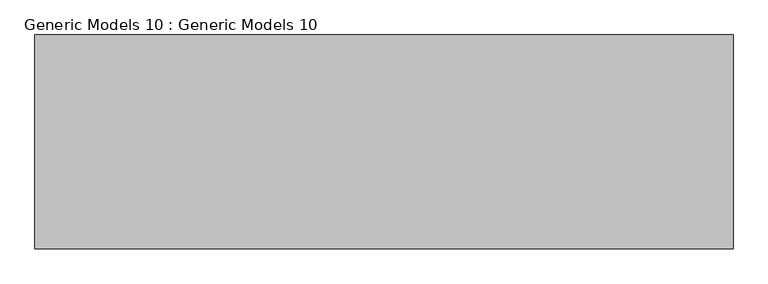
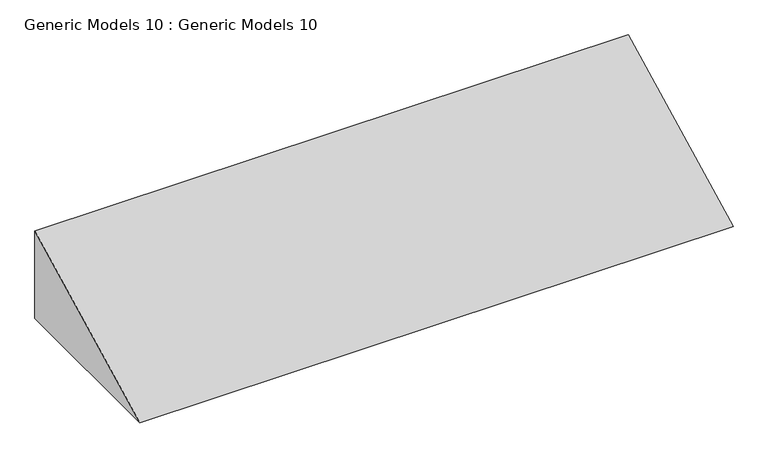
"""IFC4 building model written with IfcOpenShell, lengths in millimetres: proxy geometry, Generic Models 10 : Generic Models 10."""

from ifc_helpers import new_model, si_unit, frame, origin, place, context, project, spatial, polyline, outline, extrude, source, transform, mapped, element, save


def generic_models_10_generic_models_10_e617d169(model_context):
    return source(origin(), model_context, "Body", "SweptSolid", [
        extrude(outline(polyline([(-6795.0866303, 0.0), (-6058.4866303, 375.3164461), (-6058.4866303, 0.0), (-6795.0866303, 0.0)])), frame((1660.0362532, 0.0, 0.0), z_axis=(1.0, 0.0, 0.0), x_axis=(0.0, 1.0, 0.0)), (0.0, 0.0, 1.0), 2403.1342476),
    ])


if __name__ == "__main__":
    model = new_model("IFC4")
    model_context = context("Model", 3, world=origin())
    ifc_project = project(units=[si_unit("LENGTHUNIT", "METRE", prefix="MILLI")], contexts=[model_context])
    site = spatial("IfcSite", under=ifc_project)
    building = spatial("IfcBuilding", under=site)
    placement = place(None, origin())
    generic_models_10_generic_models_10_shape = generic_models_10_generic_models_10_e617d169(model_context)
    element("IfcBuildingElementProxy", 1, Name="Generic Models 10 : Generic Models 10", ObjectType="Generic Models 10 : Generic Models 10", at=placement, inside=building, context=model_context, shape_type="MappedRepresentation", body=[
        mapped(generic_models_10_generic_models_10_shape, transform((0.0, 0.0, 0.0), x_axis=(1.0, 0.0, 0.0), y_axis=(0.0, 1.0, 0.0), z_axis=(0.0, 0.0, 1.0))),
    ])
    save(model, "model.ifc")

# Revit data of these elements
# Element 1 (IfcBuildingElementProxy, "Generic Models 10 : Generic Models 10")
#   Materials on its faces: "Concrete, Cast-in-Place gray"
# Materials
#   "Concrete, Cast-in-Place gray": class "Concrete", colour RGB 192 192 192, transparency 0, Description = "Cast-in-place concrete", Cost = 0
